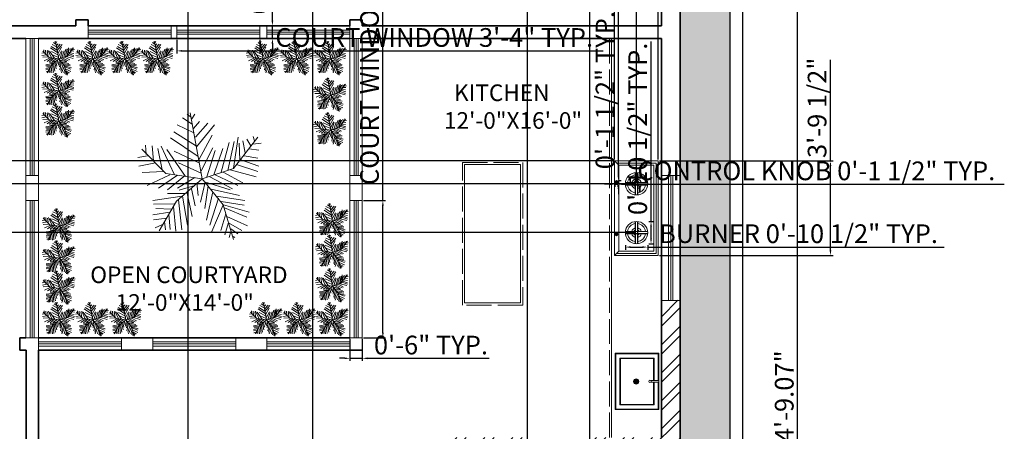
# Model space of a CAD drawing. Units: inches. Extents: x 108 to 883, y 608 to 1524.
# Tile 3 of 4: x 409 to 883, y 1040 to 1238. Entities that reach past the tile are written whole.
import ezdxf

# ---------------------------------------------------------------- set-up
doc = ezdxf.new("R2010")
doc.units = ezdxf.units.IN
doc.linetypes.add('ACAD_ISO02W100', pattern=[15, 12, -3])
for name, color, linetype, lineweight in [('A-ANNO-DIMS', 2, 'Continuous', 18), ('A-AREA-IDEN', 7, 'Continuous', 18), ('A-EQPM', 8, 'Continuous', 18), ('A-FLOR-CASE', 9, 'Continuous', 18), ('A-FLOR-CASE-HIDN', 9, 'ACAD_ISO02W100', 13), ('A-FLOR-FIXT', 9, 'Continuous', 18), ('A-WALL', 7, 'Continuous', 35), ('A-WALL-PATT', 252, 'Continuous', 13), ('C-PROP', 7, 'Continuous', 25), ('L-PLNT', 94, 'Continuous', 13)]:
    doc.layers.add(name, color=color, linetype=linetype, lineweight=lineweight)
doc.layers.add('A-GLAZ', color=244, linetype='Continuous', lineweight=18, true_color=0x991b1e)
doc.layers.add('L-PLNT-PATT', color=116, linetype='Continuous', lineweight=13, true_color=0x136734)
doc.styles.get("Standard").update_dxf_attribs({"font": 'arial.ttf'})
doc.dimstyles.new('ISO-25', dxfattribs={"dimtxt": 9, "dimasz": 2.5, "dimexe": 1.25, "dimexo": 0.625, "dimtad": 1, "dimlunit": 3, "dimtxsty": 'Standard', "dimcen": 2.5, "dimadec": 0, "dimazin": 0, "dimtfac": 1, "dimtmove": 0, "dimatfit": 3, "dimfxl": 1, "dimarcsym": 0})

# ---------------------------------------------------------------- blocks, each defined once
blk = doc.blocks.new('*U13')
for p, q in [((-8.737, 47.138), (-17.069, 52.711)), ((-10.186, 53.64), (-13.084, 55.962)), ((0, 0), (-10.5, 57)), ((-9.099, 51.782), (-6.563, 55.962)), ((-7.288, 39.707), (-21.778, 46.673)), ((-7.65, 43.423), (-2.578, 49.46)), ((-5.839, 35.992), (4.667, 48.067)), ((-5.114, 27.632), (10.463, 46.673)), ((-3.665, 19.273), (-27.574, 35.527)), ((-5.114, 28.097), (-24.676, 40.636)), ((-2.941, 16.486), (8.652, 37.85)), ((27, 9), (48, 36)), ((27.127, 9.056), (31.112, 35.992)), ((44.153, 36.456), (45.239, 32.741)), ((-48.585, 21.131), (-49.309, 29.026)), ((-43.513, 28.561), (-42.427, 15.558)), ((-38.442, 26.239), (-34.819, 7.663)), ((-35.544, 28.097), (-24.314, 3.947)), ((-1.129, 6.734), (9.014, 26.704)), ((10.101, 3.483), (17.708, 26.239)), ((16.259, 5.805), (23.142, 31.348)), ((22.055, 7.198), (27.489, 32.277)), ((31.836, 30.883), (32.561, 16.486)), ((35.096, 32.741), (37.27, 22.524)), ((38.719, 34.134), (41.979, 28.561)), ((40.53, 25.775), (48.862, 24.846)), ((43.791, 29.954), (51.036, 30.883)), ((-47.498, 19.737), (-55.83, 18.344)), ((-31.5, 4.5), (-52.5, 25.5)), ((-14.533, 2.09), (-30.834, 25.31)), ((-24.314, 23.917), (-2.941, 13.7)), ((3.942, 1.625), (11.187, 24.381)), ((36.183, 19.737), (48.137, 17.88)), ((-40.615, 13.7), (-55.105, 10.913)), ((-20.691, 13.7), (-1.129, 4.876)), ((0, 0), (27, 9)), ((29.662, 12.307), (48.137, 6.269)), ((33.285, 16.486), (48.862, 10.913)), ((-33.37, 6.269), (-52.207, 5.34)), ((-28.299, 3.483), (-47.86, -5.805)), ((-21.416, 3.018), (-38.079, -8.128)), ((0, 0), (-31.5, 4.5)), ((-15.982, 2.09), (-30.11, -9.521)), ((0, 0), (-22.5, -19.5)), ((-6.563, 1.161), (-21.416, -8.128)), ((0, 0), (18, -22.5)), ((6.478, 1.625), (26.04, -8.592)), ((11.187, 3.483), (30.749, -5.805)), ((18.07, 5.805), (35.096, -3.483)), ((24.229, 7.663), (46.688, 1.625)), ((-6.563, -5.805), (-19.967, -9.985)), ((-4.752, -3.483), (-3.665, -14.629)), ((2.493, -3.019), (-1.491, -20.202)), ((1.769, -2.555), (24.229, -9.521)), ((5.029, -6.27), (2.131, -25.775)), ((-17.431, -15.094), (-42.789, -18.809)), ((-15.257, -12.772), (-30.11, -12.772)), ((-17.069, -15.094), (-12.721, -40.172)), ((-13.446, -11.378), (-8.737, -32.741)), ((-9.461, -8.592), (-6.201, -23.453)), ((9.014, -11.378), (3.58, -35.992)), ((14.085, -16.951), (6.478, -40.172)), ((7.565, -9.056), (32.198, -14.629)), ((12.274, -15.094), (36.907, -18.809)), ((-24.314, -21.596), (-42.427, -22.06)), ((-22.5, -19.5), (-37.5, -45)), ((-25.038, -23.918), (-22.865, -45.281)), ((-20.691, -18.345), (-17.793, -44.352)), ((18.07, -22.524), (8.289, -45.745)), ((16.259, -19.738), (36.183, -22.989)), ((18, -22.5), (27, -52.5)), ((18.433, -22.524), (40.53, -29.026)), ((19.157, -25.311), (38.719, -33.206)), ((-28.299, -29.026), (-42.789, -31.348)), ((-30.834, -34.135), (-42.427, -35.528)), ((-26.849, -26.24), (-40.253, -25.775)), ((-29.023, -30.884), (-27.936, -43.887)), ((20.244, -30.419), (15.897, -44.816)), ((21.331, -32.741), (39.081, -40.636)), ((-34.457, -39.708), (-40.978, -42.494)), ((-32.646, -36.921), (-31.921, -44.352)), ((22.78, -37.85), (19.519, -48.532)), ((22.78, -38.314), (34.372, -44.816)), ((24.591, -45.745), (23.142, -50.854)), ((24.591, -43.423), (30.749, -47.603)), ((26.764, -49.925), (28.213, -50.854))]:
    blk.add_line(p, q)
blk = doc.blocks.new('*D14')
at = {"layer": 'A-ANNO-DIMS', "color": 0, "lineweight": -2, "transparency": 16777216}
for p, q in [((757.75, 1442.18), (784.93, 1442.18)), ((783.68, 667.61), (783.68, 1439.68)), ((757.75, 665.11), (784.93, 665.11))]:
    blk.add_line(p, q, dxfattribs=at)
at = {"layer": 'A-ANNO-DIMS', "color": 0, "transparency": 16777216}
for points in [[(783.26, 1439.68), (784.09, 1439.68), (783.68, 1442.18)], [(783.26, 667.61), (784.09, 667.61), (783.68, 665.11)]]:
    blk.add_solid(points, dxfattribs=at)
at = {"layer": 'Defpoints', "color": 0, "transparency": 16777216}
for p in [(757.12, 1442.18), (783.68, 1442.18), (757.12, 665.11)]:
    blk.add_point(p, dxfattribs=at)
at = {"layer": 'A-ANNO-DIMS', "color": 0, "transparency": 16777216, "insert": (778.46, 1053.64), "char_height": 9, "attachment_point": 5, "rotation": 90}
blk.add_mtext('64\'-9.07"', dxfattribs=at)
blk = doc.blocks.new('WIN-60IN-EXT')
for p, q in [((60, 5.5), (0, 5.5)), ((60, 4.5), (0, 4.5)), ((60, 3.5), (0, 3.5))]:
    blk.add_line(p, q)
blk.add_lwpolyline([(60, 9), (60, 0), (0, 0), (0, 9)], close=True)
blk = doc.blocks.new('WIN-40IN-COURT')
for p, q in [((40, 4), (0, 4)), ((40, 3), (0, 3)), ((40, 2), (0, 2))]:
    blk.add_line(p, q)
blk.add_lwpolyline([(0, 6), (40, 6), (40, 0), (0, 0)], close=True)
blk = doc.blocks.new('WIN-66IN-COURT')
for p, q in [((6, 66), (0, 66)), ((2, 66), (2, 0)), ((3, 66), (3, 0)), ((4, 66), (4, 0)), ((0, 0), (6, 0))]:
    blk.add_line(p, q)
blk = doc.blocks.new('COOKTOP-BURNER')
for p, q in [((4.77, 10.71), (4.77, 0.03)), ((4.87, 10.72), (4.87, 0.02)), ((5.87, 10.72), (5.87, 0.02)), ((5.97, 10.71), (5.97, 0.03)), ((0.02, 5.87), (10.72, 5.87)), ((0.02, 4.87), (10.72, 4.87)), ((0.03, 5.97), (10.71, 5.97)), ((0.03, 4.77), (10.71, 4.77))]:
    blk.add_line(p, q)
blk.add_circle((5.37, 5.37), 5.37)
for radius, start, end in [(4.37, 97.891, 172.109), (4.37, 7.891, 82.109), (4.37, 187.891, 262.109), (2.37, 104.6625, 165.3375), (2.37, 194.6625, 255.3375), (1.37, 115.9661, 154.0339), (1.37, 205.9661, 244.0339), (2.37, 14.6625, 75.3375), (1.37, 25.9661, 64.0339), (1.37, 295.9661, 334.0339), (2.37, 284.6625, 345.3375), (4.37, 277.891, 352.109)]:
    blk.add_arc((5.37, 5.37), radius, start, end)
blk = doc.blocks.new('COOKTOP-KNOB')
for p, q in [((0.46, 1.45), (0.46, 0.06)), ((1.06, 1.45), (1.06, 0.06))]:
    blk.add_line(p, q)
blk.add_circle((0.76, 0.76), 0.755)
for radius, start, end in [(0.555, 122.7036, 237.2964), (0.355, 147.6148, 212.3852), (0.555, 302.7036, 57.2964), (0.355, 327.6148, 32.3852)]:
    blk.add_arc((0.76, 0.76), radius, start, end)
blk = doc.blocks.new('*D26')
at = {"layer": 'A-ANNO-DIMS', "color": 0, "lineweight": -2, "transparency": 16777216}
for p, q in [((484.83, 1228.55), (484.83, 1221.93)), ((524.83, 1228.55), (524.83, 1221.93)), ((487.33, 1223.18), (522.33, 1223.18)), ((524.83, 1223.18), (690.18, 1223.18))]:
    blk.add_line(p, q, dxfattribs=at)
at = {"layer": 'A-ANNO-DIMS', "color": 0, "transparency": 16777216}
for points in [[(487.33, 1223.59), (487.33, 1222.76), (484.83, 1223.18)], [(522.33, 1223.59), (522.33, 1222.76), (524.83, 1223.18)]]:
    blk.add_solid(points, dxfattribs=at)
at = {"layer": 'Defpoints', "color": 0, "transparency": 16777216}
for p in [(484.83, 1229.18), (524.83, 1229.18), (524.83, 1223.18)]:
    blk.add_point(p, dxfattribs=at)
at = {"layer": 'A-ANNO-DIMS', "color": 0, "transparency": 16777216, "insert": (608.75, 1228.46), "char_height": 9, "attachment_point": 5}
blk.add_mtext('COURT WINDOW 3\'-4" TYP.', dxfattribs=at)
blk = doc.blocks.new('*D27')
at = {"layer": 'A-ANNO-DIMS', "color": 0, "lineweight": -2, "transparency": 16777216}
for p, q in [((530.83, 1237.68), (530.83, 1296.29)), ((525.45, 1235.18), (532.08, 1235.18)), ((530.83, 1229.18), (530.83, 1235.18)), ((525.45, 1229.18), (532.08, 1229.18)), ((530.83, 1226.68), (530.83, 1224.18))]:
    blk.add_line(p, q, dxfattribs=at)
at = {"layer": 'A-ANNO-DIMS', "color": 0, "transparency": 16777216}
for points in [[(530.41, 1237.68), (531.24, 1237.68), (530.83, 1235.18)], [(530.41, 1226.68), (531.24, 1226.68), (530.83, 1229.18)]]:
    blk.add_solid(points, dxfattribs=at)
at = {"layer": 'Defpoints', "color": 0, "transparency": 16777216}
for p in [(524.83, 1235.18), (530.83, 1235.18), (524.83, 1229.18)]:
    blk.add_point(p, dxfattribs=at)
at = {"layer": 'A-ANNO-DIMS', "color": 0, "transparency": 16777216, "insert": (525.61, 1268.23), "char_height": 9, "attachment_point": 5, "rotation": 90}
blk.add_mtext('0\'-6" TYP.', dxfattribs=at)
blk = doc.blocks.new('*D32')
at = {"layer": 'A-ANNO-DIMS', "color": 0, "lineweight": -2, "transparency": 16777216}
for p, q in [((584.02, 1151.18), (584.02, 1316.53)), ((574.75, 1151.18), (585.27, 1151.18)), ((584.02, 1087.68), (584.02, 1148.68)), ((574.75, 1085.18), (585.27, 1085.18))]:
    blk.add_line(p, q, dxfattribs=at)
at = {"layer": 'A-ANNO-DIMS', "color": 0, "transparency": 16777216}
for points in [[(583.6, 1148.68), (584.44, 1148.68), (584.02, 1151.18)], [(583.6, 1087.68), (584.44, 1087.68), (584.02, 1085.18)]]:
    blk.add_solid(points, dxfattribs=at)
at = {"layer": 'Defpoints', "color": 0, "transparency": 16777216}
for p in [(574.12, 1151.18), (584.02, 1151.18), (574.12, 1085.18)]:
    blk.add_point(p, dxfattribs=at)
at = {"layer": 'A-ANNO-DIMS', "color": 0, "transparency": 16777216, "insert": (578.74, 1235.11), "char_height": 9, "attachment_point": 5, "rotation": 90}
blk.add_mtext('COURT WINDOW 5\'-6" TYP.', dxfattribs=at)
blk = doc.blocks.new('*D33')
at = {"layer": 'A-ANNO-DIMS', "color": 0, "lineweight": -2, "transparency": 16777216}
for p, q in [((568.12, 1084.55), (568.12, 1074.03)), ((574.12, 1084.55), (574.12, 1074.03)), ((565.62, 1075.28), (563.12, 1075.28)), ((568.12, 1075.28), (574.12, 1075.28)), ((576.62, 1075.28), (635.23, 1075.28))]:
    blk.add_line(p, q, dxfattribs=at)
at = {"layer": 'A-ANNO-DIMS', "color": 0, "transparency": 16777216}
for points in [[(565.62, 1075.69), (565.62, 1074.86), (568.12, 1075.28)], [(576.62, 1075.69), (576.62, 1074.86), (574.12, 1075.28)]]:
    blk.add_solid(points, dxfattribs=at)
at = {"layer": 'Defpoints', "color": 0, "transparency": 16777216}
for p in [(568.12, 1085.18), (574.12, 1085.18), (574.12, 1075.28)]:
    blk.add_point(p, dxfattribs=at)
at = {"layer": 'A-ANNO-DIMS', "color": 0, "transparency": 16777216, "insert": (607.18, 1080.5), "char_height": 9, "attachment_point": 5}
blk.add_mtext('0\'-6" TYP.', dxfattribs=at)
blk = doc.blocks.new('*D38')
at = {"layer": 'A-ANNO-DIMS', "color": 0, "lineweight": -2, "transparency": 16777216}
for p, q in [((700.8, 1129.76), (700.8, 1127.53)), ((703.3, 1128.78), (709.04, 1128.78)), ((711.54, 1129.76), (711.54, 1127.53)), ((711.54, 1128.78), (854.3, 1128.78))]:
    blk.add_line(p, q, dxfattribs=at)
at = {"layer": 'A-ANNO-DIMS', "color": 0, "transparency": 16777216}
for points in [[(703.3, 1129.2), (703.3, 1128.36), (700.8, 1128.78)], [(709.04, 1129.2), (709.04, 1128.36), (711.54, 1128.78)]]:
    blk.add_solid(points, dxfattribs=at)
at = {"layer": 'Defpoints', "color": 0, "transparency": 16777216}
for p in [(700.8, 1130.39), (711.54, 1130.39), (711.54, 1128.78)]:
    blk.add_point(p, dxfattribs=at)
at = {"layer": 'A-ANNO-DIMS', "color": 0, "transparency": 16777216, "insert": (784.17, 1134.06), "char_height": 9, "attachment_point": 5}
blk.add_mtext('BURNER 0\'-10 1/2" TYP.', dxfattribs=at)
blk = doc.blocks.new('*D39')
at = {"layer": 'A-ANNO-DIMS', "color": 0, "lineweight": -2, "transparency": 16777216}
for p, q in [((713.15, 1141.13), (713.15, 1227.7)), ((712.17, 1141.13), (714.4, 1141.13)), ((713.15, 1132.89), (713.15, 1138.63)), ((712.17, 1130.39), (714.4, 1130.39))]:
    blk.add_line(p, q, dxfattribs=at)
at = {"layer": 'A-ANNO-DIMS', "color": 0, "transparency": 16777216}
for points in [[(712.74, 1138.63), (713.57, 1138.63), (713.15, 1141.13)], [(712.74, 1132.89), (713.57, 1132.89), (713.15, 1130.39)]]:
    blk.add_solid(points, dxfattribs=at)
at = {"layer": 'Defpoints', "color": 0, "transparency": 16777216}
for p in [(711.54, 1141.13), (713.15, 1141.13), (711.54, 1130.39)]:
    blk.add_point(p, dxfattribs=at)
at = {"layer": 'A-ANNO-DIMS', "color": 0, "transparency": 16777216, "insert": (707.88, 1185.67), "char_height": 9, "attachment_point": 5, "rotation": 90}
blk.add_mtext('0\'-10 1/2" TYP.', dxfattribs=at)
blk = doc.blocks.new('*D40')
at = {"layer": 'A-ANNO-DIMS', "color": 0, "lineweight": -2, "transparency": 16777216}
for p, q in [((693.2, 1159.01), (690.7, 1159.01)), ((695.7, 1159.01), (697.21, 1159.01)), ((695.7, 1158.62), (695.7, 1157.76)), ((697.21, 1158.62), (697.21, 1157.76)), ((699.71, 1159.01), (883.28, 1159.01))]:
    blk.add_line(p, q, dxfattribs=at)
at = {"layer": 'A-ANNO-DIMS', "color": 0, "transparency": 16777216}
for points in [[(693.2, 1159.43), (693.2, 1158.6), (695.7, 1159.01)], [(699.71, 1159.43), (699.71, 1158.6), (697.21, 1159.01)]]:
    blk.add_solid(points, dxfattribs=at)
at = {"layer": 'Defpoints', "color": 0, "transparency": 16777216}
for p in [(695.7, 1159.24), (697.21, 1159.24), (697.21, 1159.01)]:
    blk.add_point(p, dxfattribs=at)
at = {"layer": 'A-ANNO-DIMS', "color": 0, "transparency": 16777216, "insert": (792.74, 1164.3), "char_height": 9, "attachment_point": 5}
blk.add_mtext('CONTROL KNOB 0\'-1 1/2" TYP.', dxfattribs=at)
blk = doc.blocks.new('*D41')
at = {"layer": 'A-ANNO-DIMS', "color": 0, "lineweight": -2, "transparency": 16777216}
for p, q in [((697.44, 1163.25), (697.44, 1242.83)), ((697.44, 1159.24), (697.44, 1160.75)), ((697.84, 1160.75), (698.69, 1160.75)), ((697.84, 1159.24), (698.69, 1159.24)), ((697.44, 1156.74), (697.44, 1154.24))]:
    blk.add_line(p, q, dxfattribs=at)
at = {"layer": 'A-ANNO-DIMS', "color": 0, "transparency": 16777216}
for points in [[(697.02, 1163.25), (697.85, 1163.25), (697.44, 1160.75)], [(697.02, 1156.74), (697.85, 1156.74), (697.44, 1159.24)]]:
    blk.add_solid(points, dxfattribs=at)
at = {"layer": 'Defpoints', "color": 0, "transparency": 16777216}
for p in [(697.21, 1160.75), (697.21, 1159.24), (697.44, 1160.75)]:
    blk.add_point(p, dxfattribs=at)
at = {"layer": 'A-ANNO-DIMS', "color": 0, "transparency": 16777216, "insert": (692.16, 1204.29), "char_height": 9, "attachment_point": 5, "rotation": 90}
blk.add_mtext('0\'-1 1/2" TYP.', dxfattribs=at)
blk = doc.blocks.new('*D52')
at = {"layer": 'A-ANNO-DIMS', "color": 0, "lineweight": -2, "transparency": 16777216}
for p, q in [((653.67, 1031.8), (653.67, 1506.88)), ((656.17, 1505.63), (681.17, 1505.63)), ((683.67, 1031.8), (683.67, 1506.88))]:
    blk.add_line(p, q, dxfattribs=at)
at = {"layer": 'A-ANNO-DIMS', "color": 0, "transparency": 16777216}
for points in [[(656.17, 1506.04), (656.17, 1505.21), (653.67, 1505.63)], [(681.17, 1506.04), (681.17, 1505.21), (683.67, 1505.63)]]:
    blk.add_solid(points, dxfattribs=at)
at = {"layer": 'Defpoints', "color": 0, "transparency": 16777216}
for p in [(683.67, 1505.63), (653.67, 1031.18), (683.67, 1031.18)]:
    blk.add_point(p, dxfattribs=at)
at = {"layer": 'A-ANNO-DIMS', "color": 0, "transparency": 16777216, "insert": (668.67, 1510.85), "char_height": 9, "attachment_point": 5}
blk.add_mtext('2\'-6"', dxfattribs=at)
blk = doc.blocks.new('*D53')
at = {"layer": 'A-ANNO-DIMS', "color": 0, "lineweight": -2, "transparency": 16777216}
for p, q in [((490.21, 802.3), (490.21, 1506.88)), ((492.71, 1505.63), (547.71, 1505.63)), ((550.21, 802.3), (550.21, 1506.88))]:
    blk.add_line(p, q, dxfattribs=at)
at = {"layer": 'A-ANNO-DIMS', "color": 0, "transparency": 16777216}
for points in [[(492.71, 1506.04), (492.71, 1505.21), (490.21, 1505.63)], [(547.71, 1506.04), (547.71, 1505.21), (550.21, 1505.63)]]:
    blk.add_solid(points, dxfattribs=at)
at = {"layer": 'Defpoints', "color": 0, "transparency": 16777216}
for p in [(550.21, 1505.63), (490.21, 801.68), (550.21, 801.68)]:
    blk.add_point(p, dxfattribs=at)
at = {"layer": 'A-ANNO-DIMS', "color": 0, "transparency": 16777216, "insert": (520.21, 1510.85), "char_height": 9, "attachment_point": 5}
blk.add_mtext('5\'-0"', dxfattribs=at)
blk = doc.blocks.new('*D54')
at = {"layer": 'A-ANNO-DIMS', "color": 0, "lineweight": -2, "transparency": 16777216}
for p, q in [((695.57, 1170.85), (695.57, 1506.88)), ((698.07, 1505.63), (714.08, 1505.63)), ((716.58, 1170.85), (716.58, 1506.88)), ((716.58, 1505.63), (743.4, 1505.63))]:
    blk.add_line(p, q, dxfattribs=at)
at = {"layer": 'A-ANNO-DIMS', "color": 0, "transparency": 16777216}
for points in [[(698.07, 1506.04), (698.07, 1505.21), (695.57, 1505.63)], [(714.08, 1506.04), (714.08, 1505.21), (716.58, 1505.63)]]:
    blk.add_solid(points, dxfattribs=at)
at = {"layer": 'Defpoints', "color": 0, "transparency": 16777216}
for p in [(716.58, 1505.63), (695.57, 1170.23), (716.58, 1170.23)]:
    blk.add_point(p, dxfattribs=at)
at = {"layer": 'A-ANNO-DIMS', "color": 0, "transparency": 16777216, "insert": (731.24, 1510.85), "char_height": 9, "attachment_point": 5}
blk.add_mtext('1\'-9"', dxfattribs=at)
blk = doc.blocks.new('*D55')
at = {"layer": 'A-ANNO-DIMS', "color": 0, "lineweight": -2, "transparency": 16777216}
for p, q in [((799.57, 1170.23), (799.57, 1218.87)), ((717.2, 1170.23), (800.82, 1170.23)), ((799.57, 1127.26), (799.57, 1167.73)), ((717.2, 1124.76), (800.82, 1124.76))]:
    blk.add_line(p, q, dxfattribs=at)
at = {"layer": 'A-ANNO-DIMS', "color": 0, "transparency": 16777216}
for points in [[(799.15, 1167.73), (799.99, 1167.73), (799.57, 1170.23)], [(799.15, 1127.26), (799.99, 1127.26), (799.57, 1124.76)]]:
    blk.add_solid(points, dxfattribs=at)
at = {"layer": 'Defpoints', "color": 0, "transparency": 16777216}
for p in [(716.58, 1170.23), (799.57, 1170.23), (716.58, 1124.76)]:
    blk.add_point(p, dxfattribs=at)
at = {"layer": 'A-ANNO-DIMS', "color": 0, "transparency": 16777216, "insert": (794.29, 1195.8), "char_height": 9, "attachment_point": 5, "rotation": 90}
blk.add_mtext('3\'-9 1/2"', dxfattribs=at)
blk = doc.blocks.new('*D56')
at = {"layer": 'A-ANNO-DIMS', "color": 0, "lineweight": -2, "transparency": 16777216}
for p, q in [((705.55, 1159.23), (140.51, 1159.23)), ((141.76, 1156.73), (141.76, 1138.26)), ((705.55, 1135.76), (140.51, 1135.76)), ((141.76, 1135.76), (141.76, 1080.97))]:
    blk.add_line(p, q, dxfattribs=at)
at = {"layer": 'A-ANNO-DIMS', "color": 0, "transparency": 16777216}
for points in [[(141.35, 1156.73), (142.18, 1156.73), (141.76, 1159.23)], [(141.35, 1138.26), (142.18, 1138.26), (141.76, 1135.76)]]:
    blk.add_solid(points, dxfattribs=at)
at = {"layer": 'Defpoints', "color": 0, "transparency": 16777216}
for p in [(706.17, 1159.23), (141.76, 1135.76), (706.17, 1135.76)]:
    blk.add_point(p, dxfattribs=at)
at = {"layer": 'A-ANNO-DIMS', "color": 0, "transparency": 16777216, "insert": (136.48, 1107.11), "char_height": 9, "attachment_point": 5, "rotation": 90}
blk.add_mtext('1\'-11 1/2"', dxfattribs=at)
blk = doc.blocks.new('*D57')
at = {"layer": 'A-ANNO-DIMS', "color": 0, "lineweight": -2, "transparency": 16777216}
for p, q in [((694.94, 1170.23), (140.51, 1170.23)), ((141.76, 1167.73), (141.76, 1161.73)), ((705.55, 1159.23), (140.51, 1159.23)), ((141.76, 1159.23), (141.76, 1124.56))]:
    blk.add_line(p, q, dxfattribs=at)
at = {"layer": 'A-ANNO-DIMS', "color": 0, "transparency": 16777216}
for points in [[(141.35, 1167.73), (142.18, 1167.73), (141.76, 1170.23)], [(141.35, 1161.73), (142.18, 1161.73), (141.76, 1159.23)]]:
    blk.add_solid(points, dxfattribs=at)
at = {"layer": 'Defpoints', "color": 0, "transparency": 16777216}
for p in [(695.57, 1170.23), (141.76, 1159.23), (706.17, 1159.23)]:
    blk.add_point(p, dxfattribs=at)
at = {"layer": 'A-ANNO-DIMS', "color": 0, "transparency": 16777216, "insert": (136.54, 1140.64), "char_height": 9, "attachment_point": 5, "rotation": 90}
blk.add_mtext('0\'-11"', dxfattribs=at)
blk = doc.blocks.new('*D58')
at = {"layer": 'A-ANNO-DIMS', "color": 0, "lineweight": -2, "transparency": 16777216}
for p, q in [((695.57, 1170.85), (695.57, 1506.88)), ((698.07, 1505.63), (703.67, 1505.63)), ((706.17, 1159.85), (706.17, 1506.88)), ((706.17, 1505.63), (761.81, 1505.63))]:
    blk.add_line(p, q, dxfattribs=at)
at = {"layer": 'A-ANNO-DIMS', "color": 0, "transparency": 16777216}
for points in [[(698.07, 1506.04), (698.07, 1505.21), (695.57, 1505.63)], [(703.67, 1506.04), (703.67, 1505.21), (706.17, 1505.63)]]:
    blk.add_solid(points, dxfattribs=at)
at = {"layer": 'Defpoints', "color": 0, "transparency": 16777216}
for p in [(706.17, 1505.63), (695.57, 1170.23), (706.17, 1159.23)]:
    blk.add_point(p, dxfattribs=at)
at = {"layer": 'A-ANNO-DIMS', "color": 0, "transparency": 16777216, "insert": (735.24, 1510.91), "char_height": 9, "attachment_point": 5}
blk.add_mtext('0\'-10 1/2"', dxfattribs=at)

msp = doc.modelspace()

# ---------------------------------------------------------------- hatches: boundary and pattern name
at = {"layer": 'A-WALL-PATT'}
h = msp.add_hatch(dxfattribs=at)
h.set_pattern_fill('ANSI32', color=256)
h.paths.add_polyline_path([(373.121, 1085.177), (292.121, 1085.177), (292.121, 1127.011), (283.121, 1127.011), (283.121, 1085.177), (235.212, 1085.177), (235.212, 1029.423), (244.212, 1029.423), (244.212, 1079.177), (373.121, 1079.177), (373.121, 1084.577)])
h.paths.add_polyline_path([(349.212, 911.177), (244.212, 911.177), (244.212, 969.423), (235.212, 969.423), (235.212, 776.177), (266.885, 776.177), (266.885, 785.177), (244.212, 785.177), (244.212, 905.177), (316.212, 905.177), (316.212, 902.177), (322.212, 902.177), (322.212, 905.177), (349.212, 905.177)])
h.paths.add_polyline_path([(484.212, 839.177), (473.778, 839.177), (473.778, 830.177), (478.212, 830.177), (478.212, 770.177), (484.212, 770.177), (484.212, 801.677), (490.212, 801.677), (490.212, 806.177), (490.212, 807.677), (484.212, 807.677)])
h.paths.add_polyline_path([(562.212, 830.177), (566.671, 830.177), (566.671, 839.177), (556.212, 839.177), (556.212, 807.677), (550.212, 807.677), (550.212, 806.177), (550.212, 801.677), (556.212, 801.677), (556.212, 770.177), (562.212, 770.177)])
h.paths.add_polyline_path([(622.212, 848.109), (613.212, 848.109), (613.212, 839.177), (611.671, 839.177), (611.671, 830.177), (622.212, 830.177)])
h.paths.add_polyline_path([(690.201, 911.177), (619.212, 911.177), (619.212, 1031.177), (653.667, 1031.177), (653.667, 1037.177), (613.212, 1037.177), (613.212, 893.109), (622.212, 893.109), (622.212, 902.177), (690.201, 902.177)])
h.paths.add_polyline_path([(727.121, 941.177), (718.121, 941.177), (718.121, 911.177), (711.201, 911.177), (711.201, 902.177), (727.121, 902.177)])
h.paths.add_polyline_path([(727.121, 1103.177), (718.121, 1103.177), (718.121, 1037.177), (683.667, 1037.177), (683.667, 1031.177), (718.121, 1031.177), (718.121, 1001.177), (727.121, 1001.177)])
h.paths.add_polyline_path([(727.121, 1412.177), (676.121, 1412.177), (676.121, 1403.177), (718.121, 1403.177), (718.121, 1295.236), (727.121, 1295.236)])
h.paths.add_polyline_path([(574.121, 1403.177), (616.121, 1403.177), (616.121, 1412.177), (548.621, 1412.177), (548.621, 1403.177), (568.121, 1403.177), (568.121, 1307.177), (565.121, 1307.177), (565.121, 1301.177), (568.121, 1301.177), (568.121, 1274.177), (574.121, 1274.177)])
h.paths.add_polyline_path([(508.121, 1403.177), (527.621, 1403.177), (527.621, 1412.177), (483.029, 1412.177), (483.029, 1403.177), (502.121, 1403.177), (502.121, 1307.177), (475.121, 1307.177), (475.121, 1301.177), (535.121, 1301.177), (535.121, 1307.177), (508.121, 1307.177)])
h.paths.add_polyline_path([(462.029, 1412.177), (394.121, 1412.177), (394.121, 1403.177), (436.121, 1403.177), (436.121, 1274.177), (442.121, 1274.177), (442.121, 1301.177), (445.121, 1301.177), (445.121, 1307.177), (442.121, 1307.177), (442.121, 1403.177), (462.029, 1403.177)])
h.paths.add_polyline_path([(334.121, 1412.177), (283.121, 1412.177), (283.121, 1288.13), (292.121, 1288.13), (292.121, 1403.177), (334.121, 1403.177)])
at = {"layer": 'L-PLNT-PATT'}
h = msp.add_hatch(dxfattribs=at)
h.set_pattern_fill('CROSS', color=256)
h.paths.add_polyline_path([(751.121, 1436.177), (241.212, 1436.177), (241.212, 1085.177), (283.121, 1085.177), (283.121, 1412.177), (727.121, 1412.177), (727.121, 902.177), (751.121, 902.177)])

# ---------------------------------------------------------------- linework, layer by layer
at = {"layer": 'A-EQPM'}
for p, q in [((697.567, 1168.227), (695.567, 1170.227)), ((697.567, 1126.76), (695.567, 1124.76))]:
    msp.add_line(p, q, dxfattribs=at)
for points in [[(695.567, 1170.227), (716.576, 1170.227), (716.576, 1124.76), (695.567, 1124.76)], [(697.567, 1168.227), (714.576, 1168.227), (714.576, 1126.76), (697.567, 1126.76)]]:
    msp.add_lwpolyline(points, close=True, dxfattribs=at)
msp.add_lwpolyline([(696.567, 1169.227), (715.576, 1169.227), (715.576, 1125.76), (696.567, 1125.76)], dxfattribs=at)
at = {"layer": 'A-FLOR-CASE'}
msp.add_line((694.121, 1229.177), (694.121, 1037.177), dxfattribs=at)
msp.add_lwpolyline([(623.34, 1168.537), (650.368, 1168.537), (650.368, 1101.899), (623.34, 1101.899)], close=True, dxfattribs=at)
at = {"layer": 'A-FLOR-CASE-HIDN'}
msp.add_line((693.121, 1229.177), (693.121, 1037.177), dxfattribs=at)
msp.add_lwpolyline([(622.34, 1169.537), (651.368, 1169.537), (651.368, 1100.899), (622.34, 1100.899)], close=True, dxfattribs=at)
at = {"layer": 'A-FLOR-FIXT'}
for p, q in [((704.701, 1064.122), (707.263, 1064.122)), ((706.921, 1063.25), (705.044, 1064.994)), ((705.11, 1063.184), (706.855, 1065.06)), ((705.982, 1065.403), (705.982, 1062.841)), ((713.042, 1063.744), (716.891, 1063.744)), ((713.069, 1064.544), (716.891, 1064.544))]:
    msp.add_line(p, q, dxfattribs=at)
msp.add_lwpolyline([(695.894, 1077.702), (716.891, 1077.702), (716.891, 1050.586), (695.894, 1050.586)], close=True, dxfattribs=at)
for points in [[(716.591, 1063.744), (716.591, 1050.886), (696.194, 1050.886), (696.194, 1077.402), (716.591, 1077.402), (716.591, 1064.544)], [(714.591, 1063.744), (714.591, 1052.886), (698.194, 1052.886), (698.194, 1075.402), (714.591, 1075.402), (714.591, 1064.544)], [(714.391, 1063.744), (714.391, 1053.086), (698.394, 1053.086), (698.394, 1075.202), (714.391, 1075.202), (714.391, 1064.544)]]:
    msp.add_lwpolyline(points, dxfattribs=at)
for centre, radius in [((705.982, 1064.122), 1.281), ((705.982, 1064.122), 0.981), ((712.633, 1064.159), 0.582)]:
    msp.add_circle(centre, radius, dxfattribs=at)
at = {"layer": 'A-GLAZ'}
for p, q in [((412.121, 1229.177), (412.121, 1085.177)), ((418.121, 1229.177), (418.121, 1085.177)), ((568.121, 1229.177), (568.121, 1085.177)), ((574.121, 1229.177), (574.121, 1079.177))]:
    msp.add_line(p, q, dxfattribs=at)
at = {"layer": 'A-WALL'}
for p, q in [((727.121, 1412.177), (727.121, 902.177)), ((718.121, 1403.177), (718.121, 1235.177)), ((442.121, 1238.177), (436.121, 1238.177)), ((436.121, 1238.177), (436.121, 1235.177)), ((442.121, 1238.177), (442.121, 1235.177)), ((568.121, 1238.177), (574.121, 1238.177)), ((568.121, 1238.177), (568.121, 1235.177)), ((574.121, 1238.177), (574.121, 1235.177)), ((292.121, 1235.177), (436.121, 1235.177)), ((442.121, 1235.177), (568.121, 1235.177)), ((574.121, 1235.177), (718.121, 1235.177)), ((292.121, 1229.177), (412.121, 1229.177)), ((418.121, 1229.177), (442.121, 1229.177)), ((442.121, 1229.177), (568.121, 1229.177)), ((574.121, 1229.177), (718.121, 1229.177)), ((718.121, 1229.177), (718.121, 1037.177)), ((409.121, 1085.177), (409.121, 1079.177)), ((409.121, 1085.177), (412.121, 1085.177)), ((418.121, 1085.177), (436.121, 1085.177)), ((436.121, 1085.177), (568.121, 1085.177)), ((409.121, 1079.177), (412.212, 1079.177)), ((412.212, 1079.177), (412.212, 911.177)), ((418.212, 1079.177), (418.212, 839.177)), ((418.212, 1079.177), (574.121, 1079.177))]:
    msp.add_line(p, q, dxfattribs=at)
at = {"layer": 'C-PROP'}
for p, q in [((757.121, 1442.177), (757.121, 665.11)), ((751.121, 1436.177), (751.121, 671.11))]:
    msp.add_line(p, q, dxfattribs=at)

# ---------------------------------------------------------------- block references
at = {"layer": 'A-EQPM'}
for name, p in [('COOKTOP-BURNER', (700.802, 1153.857)), ('COOKTOP-KNOB', (695.701, 1159.24)), ('COOKTOP-BURNER', (700.802, 1130.39)), ('COOKTOP-KNOB', (695.701, 1134.236))]:
    msp.add_blockref(name, p, dxfattribs=at)
at = {"layer": 'A-GLAZ'}
for name, p in [('WIN-40IN-COURT', (442.121, 1229.177)), ('WIN-40IN-COURT', (484.825, 1229.177)), ('WIN-40IN-COURT', (528.121, 1229.177)), ('WIN-66IN-COURT', (412.121, 1163.177)), ('WIN-66IN-COURT', (568.121, 1163.177)), ('WIN-66IN-COURT', (412.121, 1085.177)), ('WIN-66IN-COURT', (568.121, 1085.177)), ('WIN-40IN-COURT', (418.121, 1079.177)), ('WIN-40IN-COURT', (473.229, 1079.177)), ('WIN-40IN-COURT', (528.121, 1079.177))]:
    msp.add_blockref(name, p, dxfattribs=at)
at = {"layer": 'A-GLAZ', "rotation": 90}
msp.add_blockref('WIN-60IN-EXT', (727.121, 1103.176), dxfattribs=at)
at = {"layer": 'L-PLNT'}
for p, xscale, yscale, zscale in [((427.987, 1219.324), 0.1481699113864655, 0.1481699113864655, 0.1481699113864655), ((444.4, 1219.324), 0.1481699113864655, 0.1481699113864655, 0.1481699113864655), ((459.844, 1219.324), 0.1481699113864655, 0.1481699113864655, 0.1481699113864655), ((475.607, 1219.324), 0.1481699113864655, 0.1481699113864655, 0.1481699113864655), ((526.439, 1219.324), 0.1481699113864655, 0.1481699113864655, 0.1481699113864655), ((542.625, 1219.324), 0.1481699113864655, 0.1481699113864655, 0.1481699113864655), ((558.916, 1219.324), 0.1481699113864655, 0.1481699113864655, 0.1481699113864655), ((427.987, 1203.965), 0.1481699113864655, 0.1481699113864655, 0.1481699113864655), ((558.916, 1201.814), 0.1481699113864655, 0.1481699113864655, 0.1481699113864655), ((427.987, 1189.358), 0.1481699113864655, 0.1481699113864655, 0.1481699113864655), ((497.072, 1161.668), 0.5555794383368058, 0.5555794383368058, 0.5555794383368058), ((558.916, 1185.061), 0.1481699113864655, 0.1481699113864655, 0.1481699113864655), ((559.814, 1141.326), 0.1481699113864655, 0.1481699113864655, 0.1481699113864655), ((428.233, 1138.847), 0.1481699113864655, 0.1481699113864655, 0.1481699113864655), ((559.814, 1126.246), 0.1481699113864655, 0.1481699113864655, 0.1481699113864655), ((428.233, 1123.532), 0.1481699113864655, 0.1481699113864655, 0.1481699113864655), ((428.233, 1108.927), 0.1481699113864655, 0.1481699113864655, 0.1481699113864655), ((559.814, 1110.034), 0.1481699113864655, 0.1481699113864655, 0.1481699113864655), ((428.233, 1093.762), 0.1481699113864655, 0.1481699113864655, 0.1481699113864655), ((444.267, 1093.762), 0.1481699113864655, 0.1481699113864655, 0.1481699113864655), ((460.242, 1093.762), 0.1481699113864655, 0.1481699113864655, 0.1481699113864655), ((528.008, 1093.762), 0.1481699113864655, 0.1481699113864655, 0.1481699113864655), ((544.033, 1093.762), 0.1481699113864655, 0.1481699113864655, 0.1481699113864655), ((559.814, 1093.762), 0.1481699113864655, 0.1481699113864655, 0.1481699113864655)]:
    msp.add_blockref('*U13', p, dxfattribs=dict(at, xscale=xscale, yscale=yscale, zscale=zscale))

# ---------------------------------------------------------------- texts
at = {"layer": 'A-AREA-IDEN', "char_height": 8, "attachment_point": 1}
for s, width, insert in [('  KITCHEN\\P12\'-0"X16\'-0"', 64.34246, (613.397, 1207.036)), ('OPEN COURTYARD \\P     12\'-0"X14\'-0"', 106.61645, (443.096, 1119.479))]:
    msp.add_mtext_dynamic_manual_height_columns(s, width=width, gutter_width=12.5, heights=[0], dxfattribs=dict(at, insert=insert))

# ---------------------------------------------------------------- dimensions: what is measured, and where the dimension line sits
at = {"layer": 'A-ANNO-DIMS'}
for base, p1, p2, picture, middle in [((706.173, 1505.627), (695.567, 1170.227), (706.173, 1159.227), '*D58', (735.242, 1510.905)), ((550.212, 1505.627), (490.212, 801.677), (550.212, 801.677), '*D53', (520.212, 1510.847)), ((683.667, 1505.627), (653.667, 1031.177), (683.667, 1031.177), '*D52', (668.667, 1510.847)), ((716.576, 1505.627), (695.567, 1170.227), (716.576, 1170.227), '*D54', (731.239, 1510.847))]:
    dim = msp.add_linear_dim(base=base, p1=p1, p2=p2, dimstyle='ISO-25', override={"dimdec": 1, "dimlfac": 1, "dimrnd": 0, "dimzin": 1, "dimdsep": 46, "dimlunit": 4, "dimfrac": 2}, dxfattribs=at)
    dim.commit()
    dim.dimension.update_dxf_attribs({"geometry": picture, "text_midpoint": middle})
for base, p1, p2, override, picture, middle in [((783.676, 1442.177), (757.121, 665.11), (757.121, 1442.177), {"dimclrd": 0, "dimclre": 0, "dimclrt": 0}, '*D14', (778.456, 1053.644)), ((799.571, 1170.227), (716.576, 1124.76), (716.576, 1170.227), {"dimdec": 1, "dimlfac": 1, "dimrnd": 0, "dimzin": 1, "dimdsep": 46, "dimlunit": 4, "dimfrac": 2}, '*D55', (794.29, 1195.797)), ((141.762, 1159.227), (695.567, 1170.227), (706.173, 1159.227), {"dimdec": 1, "dimlfac": 1, "dimrnd": 0, "dimzin": 1, "dimdsep": 46, "dimlunit": 4, "dimfrac": 2}, '*D57', (136.542, 1140.644)), ((141.762, 1135.76), (706.173, 1159.227), (706.173, 1135.76), {"dimdec": 1, "dimlfac": 1, "dimrnd": 0, "dimzin": 1, "dimdsep": 46, "dimlunit": 4, "dimfrac": 2}, '*D56', (136.483, 1107.115))]:
    dim = msp.add_linear_dim(base=base, p1=p1, p2=p2, angle=90, dimstyle='ISO-25', override=override, dxfattribs=at)
    dim.commit()
    dim.dimension.update_dxf_attribs({"geometry": picture, "text_midpoint": middle})
for base, p1, p2, text, picture, middle in [((584.021, 1151.177), (574.121, 1085.177), (574.121, 1151.177), 'COURT WINDOW <> TYP.', '*D32', (578.74, 1235.105)), ((530.826, 1235.177), (524.826, 1229.177), (524.826, 1235.177), '<> TYP.', '*D27', (525.605, 1268.232)), ((697.438, 1160.751), (697.211, 1159.24), (697.211, 1160.751), '<> TYP.', '*D41', (692.159, 1204.291)), ((713.154, 1141.131), (711.543, 1130.39), (711.543, 1141.131), '<> TYP.', '*D39', (707.876, 1185.667))]:
    dim = msp.add_linear_dim(base=base, p1=p1, p2=p2, angle=90, text=text, dimstyle='ISO-25', override={"dimdec": 1, "dimlfac": 1, "dimrnd": 0, "dimzin": 1, "dimdsep": 46, "dimlunit": 4, "dimfrac": 2}, dxfattribs=at)
    dim.commit()
    dim.dimension.update_dxf_attribs({"geometry": picture, "text_midpoint": middle})
for base, p1, p2, text, picture, middle in [((524.826, 1223.177), (484.826, 1229.177), (524.826, 1229.177), 'COURT WINDOW <> TYP.', '*D26', (608.754, 1228.461)), ((697.211, 1159.014), (695.701, 1159.24), (697.211, 1159.24), 'CONTROL KNOB <> TYP.', '*D40', (792.744, 1164.295)), ((711.543, 1128.779), (700.802, 1130.39), (711.543, 1130.39), 'BURNER <> TYP.', '*D38', (784.172, 1134.057)), ((574.121, 1075.277), (568.121, 1085.177), (574.121, 1085.177), '<> TYP.', '*D33', (607.176, 1080.497))]:
    dim = msp.add_linear_dim(base=base, p1=p1, p2=p2, text=text, dimstyle='ISO-25', override={"dimdec": 1, "dimlfac": 1, "dimrnd": 0, "dimzin": 1, "dimdsep": 46, "dimlunit": 4, "dimfrac": 2}, dxfattribs=at)
    dim.commit()
    dim.dimension.update_dxf_attribs({"geometry": picture, "text_midpoint": middle})

doc.saveas('drawing.dxf')
